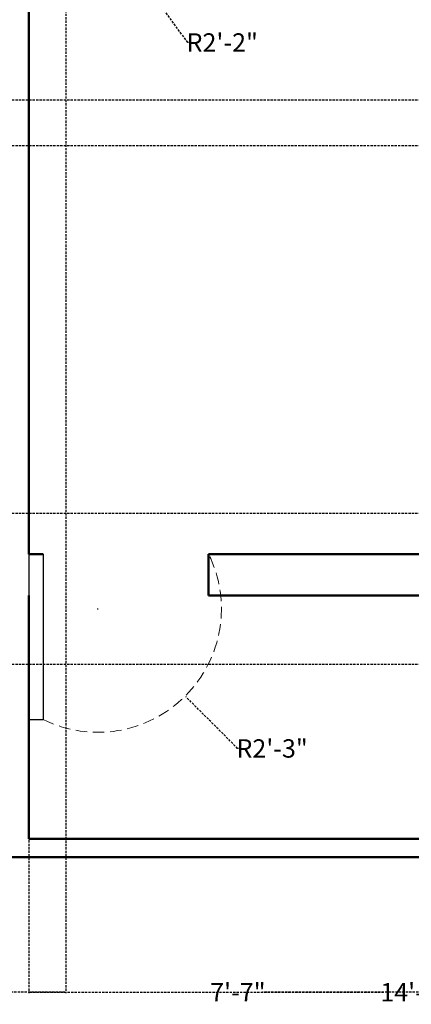
# Model space of a CAD drawing. Units: inches. Extents: x 513 to 1142, y 396 to 927.
# Tile 11 of 31: x 911 to 996, y 399 to 614. Entities that reach past the tile are written whole.
import ezdxf

# ---------------------------------------------------------------- set-up
doc = ezdxf.new("R2010")
doc.units = ezdxf.units.IN
doc.header["$MEASUREMENT"] = 0
doc.linetypes.add('DASHED', pattern=[0.75, 0.5, -0.25])
for name, color, linetype, lineweight in [('A-ANNO-DIMS', 2, 'DASHED', 18), ('A-DOOR', 4, 'Continuous', 25), ('A-DOOR-SWNG', 4, 'DASHED', 13), ('A-WALL', 7, 'Continuous', 50)]:
    doc.layers.add(name, color=color, linetype=linetype, lineweight=lineweight)
doc.styles.get("Standard").update_dxf_attribs({"font": 'arial.ttf'})
doc.dimstyles.get("Standard").update_dxf_attribs({"dimtxt": 4, "dimasz": 0.18, "dimexe": 0.18, "dimexo": 0.0625, "dimgap": 0.09, "dimtad": 0, "dimtih": 1, "dimtoh": 1, "dimdec": 0, "dimrnd": 6, "dimzin": 0, "dimdsep": 46, "dimlunit": 3, "dimtxsty": 'Standard', "dimcen": 0.09, "dimadec": 0, "dimazin": 0, "dimtfac": 1, "dimtdec": 0, "dimtofl": 0, "dimtmove": 0, "dimatfit": 3, "dimfxl": 1, "dimtolj": 1, "dimtzin": 0, "dimarcsym": 0})

# ---------------------------------------------------------------- blocks, each defined once
blk = doc.blocks.new('DOOR-LEAF-36IN')
for p, q in [((0, 0), (0, 36)), ((0, 36), (3, 36)), ((3, 36), (3, 0)), ((0, 0), (3, 0))]:
    blk.add_line(p, q)
blk = doc.blocks.new('*D137')
at = {"layer": 'A-ANNO-DIMS', "color": 0, "lineweight": -2, "transparency": 16777216}
for p, q in [((840, 770.1), (840, 401.58)), ((921, 770.07), (921, 401.58)), ((840.18, 401.76), (875.08, 401.76)), ((920.82, 401.76), (885.91, 401.76))]:
    blk.add_line(p, q, dxfattribs=at)
at = {"layer": 'A-ANNO-DIMS', "color": 0, "transparency": 16777216}
for points in [[(840.18, 401.79), (840.18, 401.73), (840, 401.76)], [(920.82, 401.79), (920.82, 401.73), (921, 401.76)]]:
    blk.add_solid(points, dxfattribs=at)
at = {"layer": 'Defpoints', "color": 0, "transparency": 16777216}
for p in [(840, 770.16), (921, 770.13), (921, 401.76)]:
    blk.add_point(p, dxfattribs=at)
at = {"layer": 'A-ANNO-DIMS', "color": 0, "transparency": 16777216, "insert": (880.5, 401.76), "char_height": 4, "attachment_point": 5}
blk.add_mtext('\\A1;6\'-9"', dxfattribs=at)
blk = doc.blocks.new('*D146')
at = {"layer": 'A-ANNO-DIMS', "color": 0, "lineweight": -2, "transparency": 16777216}
for p, q in [((913, 497.1), (913, 401.58)), ((1081, 497.1), (1081, 401.58)), ((913.18, 401.76), (990.22, 401.76)), ((1080.82, 401.76), (1003.77, 401.76))]:
    blk.add_line(p, q, dxfattribs=at)
at = {"layer": 'A-ANNO-DIMS', "color": 0, "transparency": 16777216}
for points in [[(913.18, 401.79), (913.18, 401.73), (913, 401.76)], [(1080.82, 401.79), (1080.82, 401.73), (1081, 401.76)]]:
    blk.add_solid(points, dxfattribs=at)
at = {"layer": 'Defpoints', "color": 0, "transparency": 16777216}
for p in [(913, 497.16), (1081, 497.16), (1081, 401.76)]:
    blk.add_point(p, dxfattribs=at)
at = {"layer": 'A-ANNO-DIMS', "color": 0, "transparency": 16777216, "insert": (997, 401.76), "char_height": 4, "attachment_point": 5}
blk.add_mtext('\\A1;14\'-0"', dxfattribs=at)
blk = doc.blocks.new('*D150')
at = {"layer": 'A-ANNO-DIMS', "color": 0, "lineweight": -2, "transparency": 16777216}
for p, q in [((904.06, 596.09), (1131.58, 596.09)), ((1131.4, 595.91), (1131.4, 553.23)), ((1131.4, 506.27), (1131.4, 548.96)), ((904.06, 506.09), (1131.58, 506.09))]:
    blk.add_line(p, q, dxfattribs=at)
at = {"layer": 'A-ANNO-DIMS', "color": 0, "transparency": 16777216}
for points in [[(1131.37, 595.91), (1131.43, 595.91), (1131.4, 596.09)], [(1131.37, 506.27), (1131.43, 506.27), (1131.4, 506.09)]]:
    blk.add_solid(points, dxfattribs=at)
at = {"layer": 'Defpoints', "color": 0, "transparency": 16777216}
for p in [(904, 596.09), (904, 506.09), (1131.4, 506.09)]:
    blk.add_point(p, dxfattribs=at)
at = {"layer": 'A-ANNO-DIMS', "color": 0, "transparency": 16777216, "insert": (1131.4, 551.09), "char_height": 4, "attachment_point": 5}
blk.add_mtext('\\A1;7\'-6"', dxfattribs=at)
blk = doc.blocks.new('*D158')
at = {"layer": 'A-ANNO-DIMS', "color": 0, "lineweight": -2, "transparency": 16777216}
for p, q in [((1003.92, 497.53), (1003.92, 401.58)), ((913, 497.1), (913, 401.58)), ((913.18, 401.76), (953.07, 401.76)), ((1003.74, 401.76), (963.85, 401.76))]:
    blk.add_line(p, q, dxfattribs=at)
at = {"layer": 'A-ANNO-DIMS', "color": 0, "transparency": 16777216}
for points in [[(913.18, 401.79), (913.18, 401.73), (913, 401.76)], [(1003.74, 401.79), (1003.74, 401.73), (1003.92, 401.76)]]:
    blk.add_solid(points, dxfattribs=at)
at = {"layer": 'Defpoints', "color": 0, "transparency": 16777216}
for p in [(1003.92, 497.6), (913, 497.16), (1003.92, 401.76)]:
    blk.add_point(p, dxfattribs=at)
at = {"layer": 'A-ANNO-DIMS', "color": 0, "transparency": 16777216, "insert": (958.46, 401.76), "char_height": 4, "attachment_point": 5}
blk.add_mtext('\\A1;7\'-7"', dxfattribs=at)
blk = doc.blocks.new('*D171')
at = {"layer": 'A-ANNO-DIMS', "color": 0, "lineweight": -2, "transparency": 16777216}
for p, q in [((904.06, 596.09), (1131.58, 596.09)), ((1131.4, 595.91), (1131.4, 593.23)), ((1131.4, 586.27), (1131.4, 588.96)), ((904.06, 586.09), (1131.58, 586.09))]:
    blk.add_line(p, q, dxfattribs=at)
at = {"layer": 'A-ANNO-DIMS', "color": 0, "transparency": 16777216}
for points in [[(1131.37, 595.91), (1131.43, 595.91), (1131.4, 596.09)], [(1131.37, 586.27), (1131.43, 586.27), (1131.4, 586.09)]]:
    blk.add_solid(points, dxfattribs=at)
at = {"layer": 'Defpoints', "color": 0, "transparency": 16777216}
for p in [(904, 596.09), (904, 586.09), (1131.4, 586.09)]:
    blk.add_point(p, dxfattribs=at)
at = {"layer": 'A-ANNO-DIMS', "color": 0, "transparency": 16777216, "insert": (1131.4, 591.09), "char_height": 4, "attachment_point": 5}
blk.add_mtext('\\A1;0\'-10"', dxfattribs=at)
blk = doc.blocks.new('*D172')
at = {"layer": 'A-ANNO-DIMS', "color": 0, "lineweight": -2, "transparency": 16777216}
for p, q in [((904.06, 506.09), (1131.58, 506.09)), ((1131.4, 505.91), (1131.4, 491.76)), ((1131.4, 473.34), (1131.4, 487.49)), ((904.06, 473.16), (1131.58, 473.16))]:
    blk.add_line(p, q, dxfattribs=at)
at = {"layer": 'A-ANNO-DIMS', "color": 0, "transparency": 16777216}
for points in [[(1131.37, 505.91), (1131.43, 505.91), (1131.4, 506.09)], [(1131.37, 473.34), (1131.43, 473.34), (1131.4, 473.16)]]:
    blk.add_solid(points, dxfattribs=at)
at = {"layer": 'Defpoints', "color": 0, "transparency": 16777216}
for p in [(904, 506.09), (904, 473.16), (1131.4, 473.16)]:
    blk.add_point(p, dxfattribs=at)
at = {"layer": 'A-ANNO-DIMS', "color": 0, "transparency": 16777216, "insert": (1131.4, 489.63), "char_height": 4, "attachment_point": 5}
blk.add_mtext('\\A1;2\'-9"', dxfattribs=at)
blk = doc.blocks.new('*D173')
at = {"layer": 'A-ANNO-DIMS', "color": 0, "lineweight": -2, "transparency": 16777216}
for p, q in [((904.06, 637.16), (1131.58, 637.16)), ((1131.4, 636.98), (1131.4, 618.76)), ((1131.4, 596.27), (1131.4, 614.49)), ((904.06, 596.09), (1131.58, 596.09))]:
    blk.add_line(p, q, dxfattribs=at)
at = {"layer": 'A-ANNO-DIMS', "color": 0, "transparency": 16777216}
for points in [[(1131.37, 636.98), (1131.43, 636.98), (1131.4, 637.16)], [(1131.37, 596.27), (1131.43, 596.27), (1131.4, 596.09)]]:
    blk.add_solid(points, dxfattribs=at)
at = {"layer": 'Defpoints', "color": 0, "transparency": 16777216}
for p in [(904, 637.16), (1131.4, 637.16), (904, 596.09)]:
    blk.add_point(p, dxfattribs=at)
at = {"layer": 'A-ANNO-DIMS', "color": 0, "transparency": 16777216, "insert": (1131.4, 616.63), "char_height": 4, "attachment_point": 5}
blk.add_mtext('\\A1;3\'-5"', dxfattribs=at)
blk = doc.blocks.new('*D179')
at = {"layer": 'A-ANNO-DIMS', "color": 0, "lineweight": -2, "transparency": 16777216}
for p, q in [((927.92, 485.23), (928.1, 485.23)), ((928.01, 485.14), (928.01, 485.32)), ((958.41, 454.84), (947.14, 466.11)), ((958.59, 454.84), (958.41, 454.84))]:
    blk.add_line(p, q, dxfattribs=at)
at = {"layer": 'A-ANNO-DIMS', "color": 0, "transparency": 16777216}
blk.add_solid([(947.16, 466.13), (947.11, 466.09), (947.01, 466.24)], dxfattribs=at)
at = {"layer": 'Defpoints', "color": 0, "transparency": 16777216}
for p in [(928.01, 485.23), (947.01, 466.24)]:
    blk.add_point(p, dxfattribs=at)
at = {"layer": 'A-ANNO-DIMS', "color": 0, "transparency": 16777216, "insert": (965.91, 454.84), "char_height": 4, "attachment_point": 5}
blk.add_mtext('\\A1;R2\'-3"', dxfattribs=at)
blk = doc.blocks.new('*D180')
at = {"layer": 'A-ANNO-DIMS', "color": 0, "lineweight": -2, "transparency": 16777216}
for p, q in [((922.75, 642.37), (922.93, 642.37)), ((922.84, 642.28), (922.84, 642.46)), ((947.56, 608.55), (938.4, 621.09)), ((947.74, 608.55), (947.56, 608.55))]:
    blk.add_line(p, q, dxfattribs=at)
at = {"layer": 'A-ANNO-DIMS', "color": 0, "transparency": 16777216}
blk.add_solid([(938.42, 621.11), (938.37, 621.07), (938.29, 621.24)], dxfattribs=at)
at = {"layer": 'Defpoints', "color": 0, "transparency": 16777216}
for p in [(922.84, 642.37), (938.29, 621.24)]:
    blk.add_point(p, dxfattribs=at)
at = {"layer": 'A-ANNO-DIMS', "color": 0, "transparency": 16777216, "insert": (955.06, 608.55), "char_height": 4, "attachment_point": 5}
blk.add_mtext('\\A1;R2\'-2"', dxfattribs=at)

msp = doc.modelspace()

# ---------------------------------------------------------------- linework, layer by layer
at = {"layer": 'A-DOOR-SWNG', "ltscale": 5}
msp.add_arc((928.01, 485.23), 26.87, 243.6504, 26.3496, dxfattribs=at)
at = {"layer": 'A-WALL'}
for p, q in [((913, 497.16), (913, 641.16)), ((913, 497.16), (916.09, 497.16)), ((952.09, 497.16), (952.09, 488.16)), ((952.09, 497.16), (1081, 497.16)), ((913, 435.16), (913, 488.16)), ((913, 488.16), (913.09, 488.16)), ((952.09, 488.16), (1086, 488.16)), ((913, 435.16), (1086, 435.16)), ((909, 431.16), (1090, 431.16))]:
    msp.add_line(p, q, dxfattribs=at)

# ---------------------------------------------------------------- block references
at = {"layer": 'A-DOOR'}
msp.add_blockref('DOOR-LEAF-36IN', (913.08, 461.16), dxfattribs=at)

# ---------------------------------------------------------------- dimensions: what is measured, and where the dimension line sits
at = {"layer": 'A-ANNO-DIMS'}
for base, p1, p2, picture, middle in [((921, 401.76), (840, 770.16), (921, 770.13), '*D137', (880.5, 401.76)), ((1003.92, 401.76), (913, 497.16), (1003.92, 497.6), '*D158', (958.46, 401.76)), ((1081, 401.76), (913, 497.16), (1081, 497.16), '*D146', (997, 401.76))]:
    dim = msp.add_linear_dim(base=base, p1=p1, p2=p2, dimstyle='Standard', override={"dimdec": 1, "dimlfac": 1, "dimrnd": 0, "dimzin": 1, "dimdsep": 46, "dimlunit": 4, "dimfrac": 2}, dxfattribs=at)
    dim.commit()
    dim.dimension.update_dxf_attribs({"geometry": picture, "text_midpoint": middle})
for center, mpoint, picture, middle in [((922.84, 642.37), (938.29, 621.24), '*D180', (955.06, 608.55)), ((928.01, 485.23), (947.01, 466.24), '*D179', (965.91, 454.84))]:
    dim = msp.add_radius_dim(center=center, mpoint=mpoint, dimstyle='Standard', override={"dimdec": 1, "dimlfac": 1, "dimrnd": 0, "dimzin": 1, "dimdsep": 46, "dimlunit": 4, "dimfrac": 2}, dxfattribs=at)
    dim.commit()
    dim.dimension.update_dxf_attribs({"geometry": picture, "text_midpoint": middle, "dimtype": 164})
for base, p1, p2, picture, middle in [((1131.4, 637.16), (904, 596.09), (904, 637.16), '*D173', (1131.4, 616.63)), ((1131.4, 506.09), (904, 596.09), (904, 506.09), '*D150', (1131.4, 551.09)), ((1131.4, 586.09), (904, 596.09), (904, 586.09), '*D171', (1131.4, 591.09)), ((1131.4, 473.16), (904, 506.09), (904, 473.16), '*D172', (1131.4, 489.63))]:
    dim = msp.add_linear_dim(base=base, p1=p1, p2=p2, angle=90, dimstyle='Standard', override={"dimdec": 1, "dimlfac": 1, "dimrnd": 0, "dimzin": 1, "dimdsep": 46, "dimlunit": 4, "dimfrac": 2}, dxfattribs=at)
    dim.commit()
    dim.dimension.update_dxf_attribs({"geometry": picture, "text_midpoint": middle})

doc.saveas('drawing.dxf')
